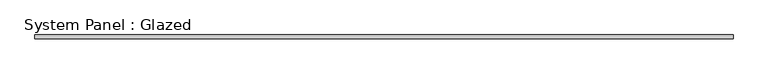
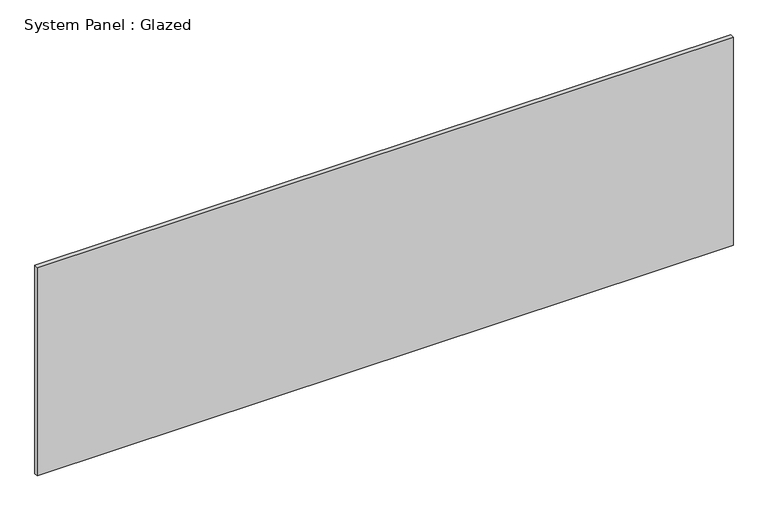
"""IFC4 building model written with IfcOpenShell, lengths in millimetres: plate geometry, System Panel : Glazed."""

from ifc_helpers import new_model, si_unit, origin, origin_with_axes, place, context, project, spatial, polyline, outline, extrude, source, transform, mapped, element, save


def system_panel_glazed_21f26c1a(model_context):
    return source(origin(), model_context, "Body", "SweptSolid", [
        extrude(outline(polyline([(2308.225, 19.05), (-2308.225, 19.05), (-2308.225, 44.45), (2308.225, 44.45), (2308.225, 19.05)])), origin_with_axes(), (0.0, 0.0, 1.0), 1460.5),
    ])


if __name__ == "__main__":
    model = new_model("IFC4")
    model_context = context("Model", 3, world=origin())
    ifc_project = project(units=[si_unit("LENGTHUNIT", "METRE", prefix="MILLI")], contexts=[model_context])
    site = spatial("IfcSite", under=ifc_project)
    building = spatial("IfcBuilding", under=site)
    placement = place(None, origin())
    system_panel_glazed_shape = system_panel_glazed_21f26c1a(model_context)
    element("IfcPlate", 1, ObjectType="System Panel : Glazed", at=placement, inside=building, context=model_context, shape_type="MappedRepresentation", body=[
        mapped(system_panel_glazed_shape, transform((0.0, 0.0, 0.0), x_axis=(1.0, 0.0, 0.0), y_axis=(0.0, 1.0, 0.0), z_axis=(0.0, 0.0, 1.0))),
    ])
    save(model, "model.ifc")

# Revit data of these elements
# Type "System Panel : Glazed"
#   Construction Type Id = "GSP4R"
#   Analytic Construction = "1/8 in Pilkington single glazing"
#   Visual Light Transmittance = 0.9
#   Solar Heat Gain Coefficient = 0.86
#   Heat Transfer Coefficient (U) = 1.18115 BTU/(h·ft²·°F)
# Element 1 (IfcPlate, "System Panel : Glazed")
#   Materials on its faces: "Glass"
# Materials
#   "Glass": class "Glass", colour RGB 0 128 192, transparency 0.75, Description = "Soda Lime Glass", Cost = 0
